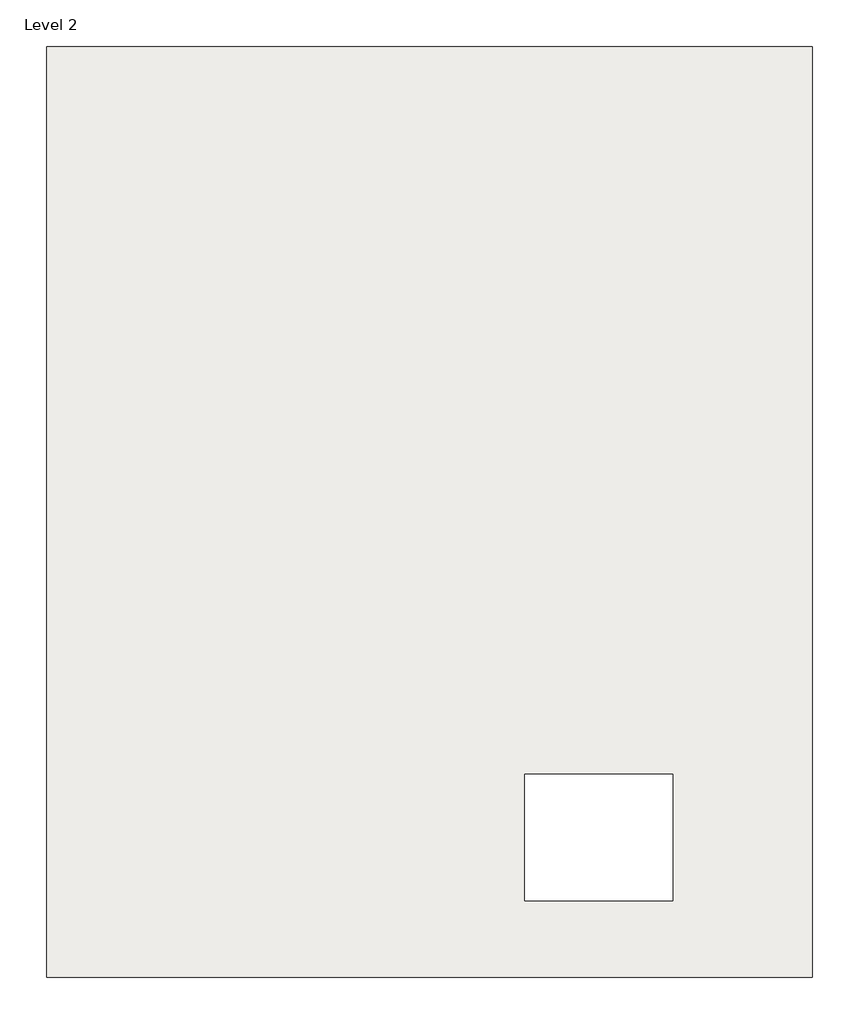
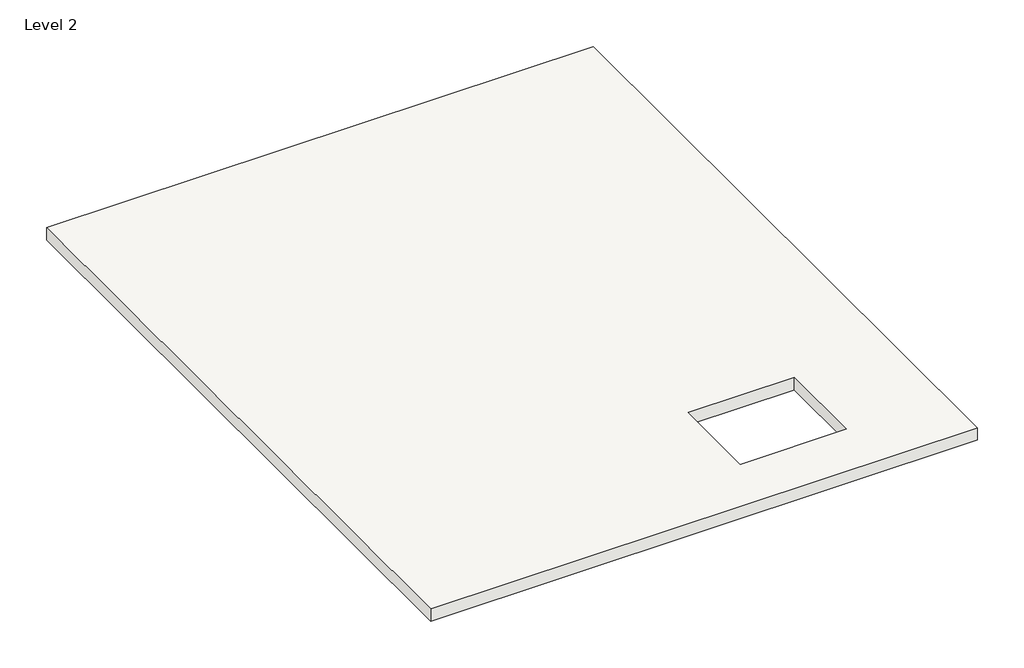
# One storey: 1 roof.
"""IFC4 building model written with IfcOpenShell, lengths in millimetres."""

from ifc_helpers import new_model, si_unit, frame, origin, place, context, project, spatial, polyline, outline, extrude, element, save

model = new_model("IFC4")

# Units and contexts
model_context = context("Model", 3, world=origin())
ifc_project = project(units=[si_unit("LENGTHUNIT", "METRE", prefix="MILLI")], contexts=[model_context])

# Site, building, storey
site = spatial("IfcSite", under=ifc_project)
building = spatial("IfcBuilding", under=site)
storey = spatial("IfcBuildingStorey", under=building, Name="Level 2", Elevation=3048.0)

# Roof
placement = place(None, origin())
element("IfcRoof", 1, ObjectType="Generic - 12\"", at=placement, inside=storey, context=model_context, shape_type="SweptSolid", body=[
    extrude(outline(polyline([(-12421.2254019, 13336.5007235), (278.7745981, 13336.5007235), (278.7745981, -2106.6992765), (-12421.2254019, -2106.6992765), (-12421.2254019, 13336.5007235)]), holes=[polyline([(-2034.156544, -831.4121747), (-2034.156544, 1261.3412642), (-4489.034821, 1261.3412642), (-4489.034821, -831.4121747), (-2034.156544, -831.4121747)])]), frame((0.0, 0.0, 3048.0), z_axis=(0.0, 0.0, 1.0), x_axis=(1.0, 0.0, 0.0)), (0.0, 0.0, 1.0), 304.8),
])

save(model, "model.ifc")

# Revit data of these elements
# Type "Generic - 12\""
#   Assembly Code = "B1020"
#   Layers, outside or top first: 1' - 0" "Brick, Soldier Course" (function 1)
# Element 1 (IfcRoof, "Generic - 12\"")
#   built-in parameter 1001705 = 11 (stored number, unit not read)
#   built-in parameter 1001710 = 33615
#   Phase Created = New Construction
#   Materials on its faces: "Brick, Soldier Course"
# Materials
#   "Brick, Soldier Course": class "Masonry", colour RGB 170 98 104, transparency 0, Description = "Common brick soldier coursed", Cost = 0
